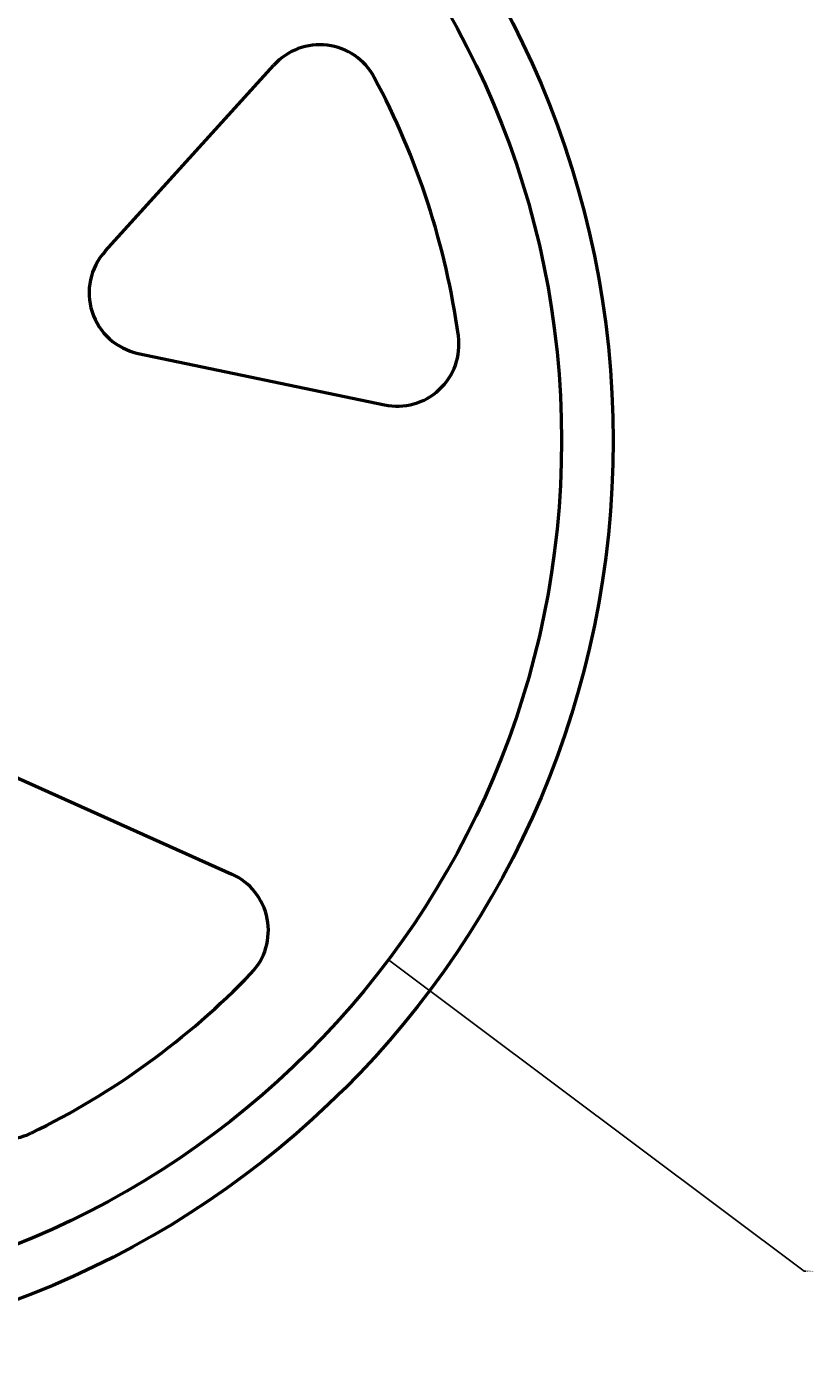
# Model space of a CAD drawing. Units: inches. Extents: x -99 to 284, y -92 to 134.
# Tile 7 of 16: x 64 to 140, y -74 to 55. Entities that reach past the tile are written whole.
import ezdxf

# ---------------------------------------------------------------- set-up
doc = ezdxf.new("R2010")
doc.units = ezdxf.units.IN
doc.header["$MEASUREMENT"] = 0
doc.layers.add('M-DIMS', color=2, linetype='Continuous', lineweight=18)
doc.layers.add('M-OUTL', color=7, linetype='Continuous', lineweight=50)
doc.styles.get("Standard").update_dxf_attribs({"font": 'arial.ttf'})
doc.dimstyles.get("Standard").update_dxf_attribs({"dimtxt": 0.18, "dimasz": 0.18, "dimexe": 0.18, "dimexo": 0.0625, "dimgap": 0.09, "dimtad": 0, "dimtih": 1, "dimtoh": 1, "dimdec": 4, "dimzin": 0, "dimdsep": 46, "dimtxsty": 'Standard', "dimcen": 0.09, "dimadec": 0, "dimazin": 0, "dimtfac": 1, "dimtdec": 4, "dimtofl": 0, "dimtmove": 0, "dimatfit": 3, "dimfxl": 1, "dimtolj": 1, "dimtzin": 0, "dimarcsym": 0})

# ---------------------------------------------------------------- blocks, each defined once
blk = doc.blocks.new('*U1')
for p, q in [((-5.21, -13.52), (-17.34, 7.65)), ((5.21, -13.52), (17.34, 7.65))]:
    blk.add_line(p, q)
for centre, start, end in [((-12.14, 10.63), 100.177, 209.8264), ((12.14, 10.63), 330.1736, 79.823), ((0, -10.54), 209.8264, 330.1736)]:
    blk.add_arc(centre, 6, start, end)
blk = doc.blocks.new('*U2')
at = {"layer": 'M-OUTL', "color": 0, "linetype": 'ByBlock', "lineweight": -2, "transparency": 16777216}
for p, rotation in [((86.16, 32.46), 288), ((65.46, -31.24), 216)]:
    blk.add_blockref('*U1', p, dxfattribs=dict(at, rotation=rotation))
blk = doc.blocks.new('*D19')
at = {"layer": 'Defpoints', "color": 0, "transparency": 16777216}
for p in [(112.98, 51.72), (-49.03, -22.01)]:
    blk.add_point(p, dxfattribs=at)
at = {"layer": 'M-DIMS', "color": 0, "lineweight": -2, "transparency": 16777216}
for p, q in [((31.89, 14.85), (32.07, 14.85)), ((31.98, 14.76), (31.98, 14.94)), ((-97.63, -44.13), (-49.19, -22.09)), ((-97.81, -44.13), (-97.63, -44.13))]:
    blk.add_line(p, q, dxfattribs=at)
at = {"layer": 'M-DIMS', "color": 0, "transparency": 16777216}
blk.add_solid([(-49.2, -22.06), (-49.18, -22.11), (-49.03, -22.01)], dxfattribs=at)
at = {"layer": 'M-DIMS', "color": 0, "transparency": 16777216, "insert": (-98.2, -44.13), "char_height": 0.18, "attachment_point": 5}
blk.add_mtext('\\A1;∅178', dxfattribs=at)
blk = doc.blocks.new('*D20')
at = {"layer": 'Defpoints', "color": 0, "transparency": 16777216}
for p in [(-35.23, 65.25), (99.18, -35.54)]:
    blk.add_point(p, dxfattribs=at)
at = {"layer": 'M-DIMS', "color": 0, "lineweight": -2, "transparency": 16777216}
for p, q in [((31.89, 14.85), (32.07, 14.85)), ((31.98, 14.76), (31.98, 14.94)), ((139.51, -65.77), (99.33, -35.65)), ((139.69, -65.77), (139.51, -65.77))]:
    blk.add_line(p, q, dxfattribs=at)
at = {"layer": 'M-DIMS', "color": 0, "transparency": 16777216}
blk.add_solid([(99.35, -35.62), (99.31, -35.67), (99.18, -35.54)], dxfattribs=at)
at = {"layer": 'M-DIMS', "color": 0, "transparency": 16777216, "insert": (140.07, -65.77), "char_height": 0.18, "attachment_point": 5}
blk.add_mtext('\\A1;∅168', dxfattribs=at)

msp = doc.modelspace()

# ---------------------------------------------------------------- linework, layer by layer
at = {"layer": 'M-OUTL'}
for radius in [89, 84]:
    msp.add_circle((31.9765, 14.8539), radius, dxfattribs=at)
for start, end in [(7.823035, 28.176965), (295.823035, 316.176965)]:
    msp.add_arc((31.9765, 14.8539), 74.6806, start, end, dxfattribs=at)

# ---------------------------------------------------------------- block references
msp.add_blockref('*U2', (0, 0), dxfattribs=at)

# ---------------------------------------------------------------- dimensions: what is measured, and where the dimension line sits
at = {"layer": 'M-DIMS'}
for p1, p2, picture, middle in [((-35.2301, 65.2451), (99.1831, -35.5373), '*D20', (140.074, -65.772)), ((112.9816, 51.7208), (-49.0286, -22.013), '*D19', (-98.1987, -44.1332))]:
    dim = msp.add_diameter_dim_2p(p1=p1, p2=p2, dimstyle='Standard', override={"dimdec": 0, "dimlfac": 1, "dimrnd": 0, "dimzin": 0, "dimdsep": 46, "dimlunit": 2}, dxfattribs=at)
    dim.commit()
    dim.dimension.update_dxf_attribs({"geometry": picture, "text_midpoint": middle, "dimtype": 163})

doc.saveas('drawing.dxf')
